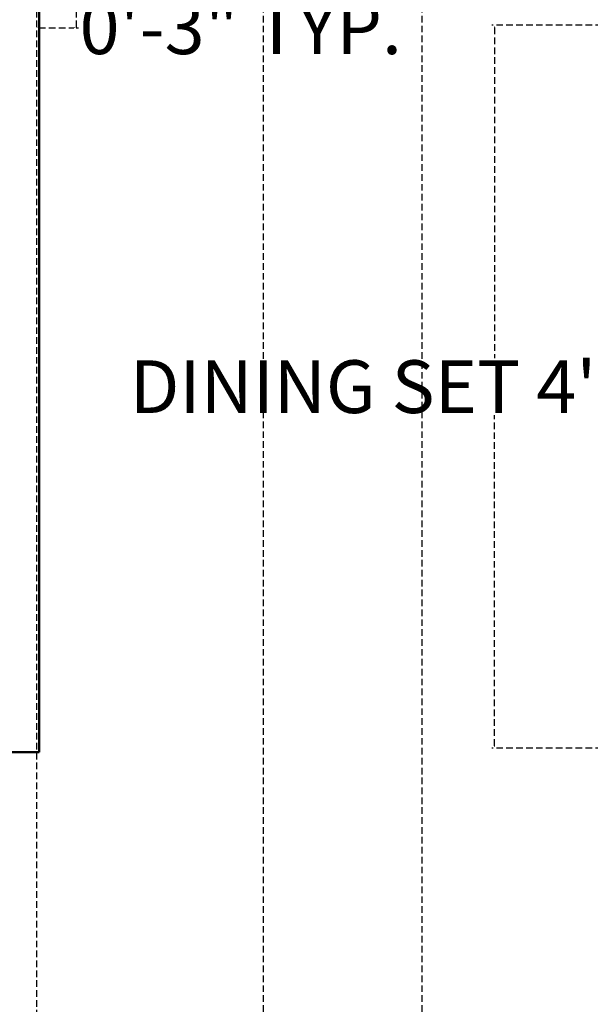
# Model space of a CAD drawing. Units: inches. Extents: x 513 to 1142, y 396 to 927.
# Tile 15 of 31: x 743 to 786, y 691 to 766. Entities that reach past the tile are written whole.
import ezdxf

# ---------------------------------------------------------------- set-up
doc = ezdxf.new("R2010")
doc.units = ezdxf.units.IN
doc.header["$MEASUREMENT"] = 0
doc.linetypes.add('DASHED', pattern=[0.75, 0.5, -0.25])
doc.layers.add('A-ANNO-DIMS', color=2, linetype='DASHED', lineweight=18)
doc.layers.add('A-WALL', color=7, linetype='Continuous', lineweight=50)
doc.styles.get("Standard").update_dxf_attribs({"font": 'arial.ttf'})
doc.dimstyles.get("Standard").update_dxf_attribs({"dimtxt": 4, "dimasz": 0.18, "dimexe": 0.18, "dimexo": 0.0625, "dimgap": 0.09, "dimtad": 0, "dimtih": 1, "dimtoh": 1, "dimdec": 0, "dimrnd": 6, "dimzin": 0, "dimdsep": 46, "dimlunit": 3, "dimtxsty": 'Standard', "dimcen": 0.09, "dimadec": 0, "dimazin": 0, "dimtfac": 1, "dimtdec": 0, "dimtofl": 0, "dimtmove": 0, "dimatfit": 3, "dimfxl": 1, "dimtolj": 1, "dimtzin": 0, "dimarcsym": 0})

# ---------------------------------------------------------------- blocks, each defined once
blk = doc.blocks.new('*D121')
at = {"layer": 'A-ANNO-DIMS', "color": 0, "lineweight": -2, "transparency": 16777216}
for p, q in [((786.62, 765.256), (778.284, 765.256)), ((778.464, 765.076), (778.464, 740.017)), ((778.464, 710.643), (778.464, 735.701)), ((786.62, 710.463), (778.284, 710.463))]:
    blk.add_line(p, q, dxfattribs=at)
at = {"layer": 'A-ANNO-DIMS', "color": 0, "transparency": 16777216}
for points in [[(778.434, 765.076), (778.494, 765.076), (778.464, 765.256)], [(778.434, 710.643), (778.494, 710.643), (778.464, 710.463)]]:
    blk.add_solid(points, dxfattribs=at)
at = {"layer": 'Defpoints', "color": 0, "transparency": 16777216}
for p in [(778.464, 765.256), (786.683, 765.256), (786.683, 710.463)]:
    blk.add_point(p, dxfattribs=at)
at = {"layer": 'A-ANNO-DIMS', "color": 0, "transparency": 16777216, "insert": (778.464, 737.859), "char_height": 4, "attachment_point": 5}
blk.add_mtext('\\A1;DINING SET 4\'-7" TYP.', dxfattribs=at)
blk = doc.blocks.new('*D124')
at = {"layer": 'A-ANNO-DIMS', "color": 0, "lineweight": -2, "transparency": 16777216}
for p, q in [((743.802, 768.607), (743.802, 764.89)), ((746.802, 768.607), (746.802, 764.89)), ((743.982, 765.07), (746.622, 765.07)), ((746.802, 765.07), (746.982, 765.07))]:
    blk.add_line(p, q, dxfattribs=at)
at = {"layer": 'A-ANNO-DIMS', "color": 0, "transparency": 16777216}
for points in [[(743.982, 765.1), (743.982, 765.04), (743.802, 765.07)], [(746.622, 765.1), (746.622, 765.04), (746.802, 765.07)]]:
    blk.add_solid(points, dxfattribs=at)
at = {"layer": 'Defpoints', "color": 0, "transparency": 16777216}
for p in [(743.802, 768.67), (746.802, 768.67), (746.802, 765.07)]:
    blk.add_point(p, dxfattribs=at)
at = {"layer": 'A-ANNO-DIMS', "color": 0, "transparency": 16777216, "insert": (759.263, 765.07), "char_height": 4, "attachment_point": 5}
blk.add_mtext('\\A1;0\'-3" TYP.', dxfattribs=at)
blk = doc.blocks.new('*D136')
at = {"layer": 'A-ANNO-DIMS', "color": 0, "lineweight": -2, "transparency": 16777216}
for p, q in [((835.995, 770.096), (835.995, 401.578)), ((743.802, 768.607), (743.802, 401.578)), ((743.982, 401.758), (784.509, 401.758)), ((835.815, 401.758), (795.289, 401.758))]:
    blk.add_line(p, q, dxfattribs=at)
at = {"layer": 'A-ANNO-DIMS', "color": 0, "transparency": 16777216}
for points in [[(743.982, 401.788), (743.982, 401.728), (743.802, 401.758)], [(835.815, 401.788), (835.815, 401.728), (835.995, 401.758)]]:
    blk.add_solid(points, dxfattribs=at)
at = {"layer": 'Defpoints', "color": 0, "transparency": 16777216}
for p in [(835.995, 770.158), (743.802, 768.67), (835.995, 401.758)]:
    blk.add_point(p, dxfattribs=at)
at = {"layer": 'A-ANNO-DIMS', "color": 0, "transparency": 16777216, "insert": (789.899, 401.758), "char_height": 4, "attachment_point": 5}
blk.add_mtext('\\A1;7\'-8"', dxfattribs=at)
blk = doc.blocks.new('*D167')
at = {"layer": 'A-ANNO-DIMS', "color": 0, "lineweight": -2, "transparency": 16777216}
for p, q in [((760.995, 637.221), (760.995, 920.738)), ((761.175, 920.558), (761.777, 920.558)), ((772.815, 920.558), (772.214, 920.558)), ((772.995, 637.221), (772.995, 920.738))]:
    blk.add_line(p, q, dxfattribs=at)
at = {"layer": 'A-ANNO-DIMS', "color": 0, "transparency": 16777216}
for points in [[(761.175, 920.588), (761.175, 920.528), (760.995, 920.558)], [(772.815, 920.588), (772.815, 920.528), (772.995, 920.558)]]:
    blk.add_solid(points, dxfattribs=at)
at = {"layer": 'Defpoints', "color": 0, "transparency": 16777216}
for p in [(772.995, 920.558), (760.995, 637.158), (772.995, 637.158)]:
    blk.add_point(p, dxfattribs=at)
at = {"layer": 'A-ANNO-DIMS', "color": 0, "transparency": 16777216, "insert": (766.995, 920.558), "char_height": 4, "attachment_point": 5}
blk.add_mtext('\\A1;1\'-0"', dxfattribs=at)
blk = doc.blocks.new('*D175')
at = {"layer": 'A-ANNO-DIMS', "color": 0, "lineweight": -2, "transparency": 16777216}
for p, q in [((772.995, 637.221), (772.995, 920.738)), ((773.175, 920.558), (793.008, 920.558)), ((823.815, 920.558), (803.982, 920.558)), ((823.995, 637.221), (823.995, 920.738))]:
    blk.add_line(p, q, dxfattribs=at)
at = {"layer": 'A-ANNO-DIMS', "color": 0, "transparency": 16777216}
for points in [[(773.175, 920.588), (773.175, 920.528), (772.995, 920.558)], [(823.815, 920.588), (823.815, 920.528), (823.995, 920.558)]]:
    blk.add_solid(points, dxfattribs=at)
at = {"layer": 'Defpoints', "color": 0, "transparency": 16777216}
for p in [(823.995, 920.558), (772.995, 637.158), (823.995, 637.158)]:
    blk.add_point(p, dxfattribs=at)
at = {"layer": 'A-ANNO-DIMS', "color": 0, "transparency": 16777216, "insert": (798.495, 920.558), "char_height": 4, "attachment_point": 5}
blk.add_mtext('\\A1;4\'-3"', dxfattribs=at)

msp = doc.modelspace()

# ---------------------------------------------------------------- linework, layer by layer
at = {"layer": 'A-WALL'}
for p, q in [((743.995, 870.158), (743.995, 710.158)), ((743.995, 710.158), (739.995, 710.158))]:
    msp.add_line(p, q, dxfattribs=at)

# ---------------------------------------------------------------- dimensions: what is measured, and where the dimension line sits
at = {"layer": 'A-ANNO-DIMS'}
for base, p1, p2, picture, middle in [((772.995, 920.558), (760.995, 637.158), (772.995, 637.158), '*D167', (766.995, 920.558)), ((823.995, 920.558), (772.995, 637.158), (823.995, 637.158), '*D175', (798.495, 920.558)), ((835.995, 401.758), (743.802, 768.67), (835.995, 770.158), '*D136', (789.899, 401.758))]:
    dim = msp.add_linear_dim(base=base, p1=p1, p2=p2, dimstyle='Standard', override={"dimdec": 1, "dimlfac": 1, "dimrnd": 0, "dimzin": 1, "dimdsep": 46, "dimlunit": 4, "dimfrac": 2}, dxfattribs=at)
    dim.commit()
    dim.dimension.update_dxf_attribs({"geometry": picture, "text_midpoint": middle})
dim = msp.add_linear_dim(base=(746.802, 765.07), p1=(743.802, 768.67), p2=(746.802, 768.67), text='<> TYP.', dimstyle='Standard', override={"dimdec": 1, "dimlfac": 1, "dimrnd": 0, "dimzin": 1, "dimdsep": 46, "dimlunit": 4, "dimfrac": 2}, dxfattribs=at)
dim.commit()
dim.dimension.update_dxf_attribs({"geometry": '*D124', "text_midpoint": (759.263, 765.07)})
dim = msp.add_linear_dim(base=(778.464, 765.256), p1=(786.683, 710.463), p2=(786.683, 765.256), angle=90, text='DINING SET <> TYP.', dimstyle='Standard', override={"dimdec": 1, "dimlfac": 1, "dimrnd": 0, "dimzin": 1, "dimdsep": 46, "dimlunit": 4, "dimfrac": 2}, dxfattribs=at)
dim.commit()
dim.dimension.update_dxf_attribs({"geometry": '*D121', "text_midpoint": (778.464, 737.859)})

doc.saveas('drawing.dxf')
